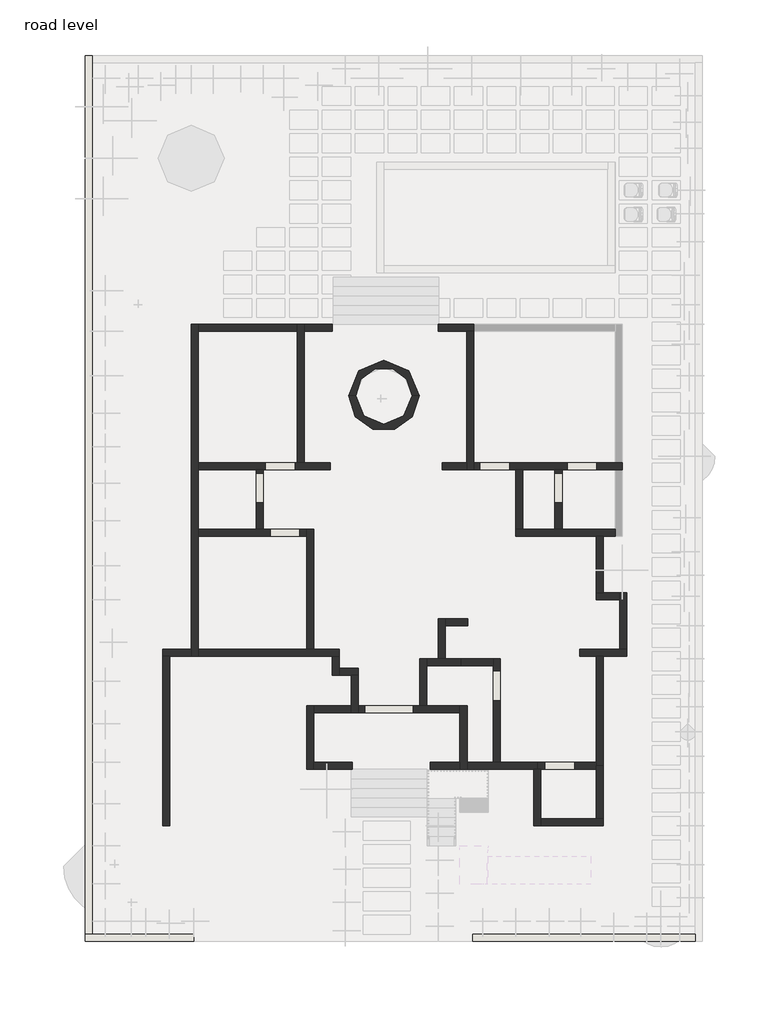
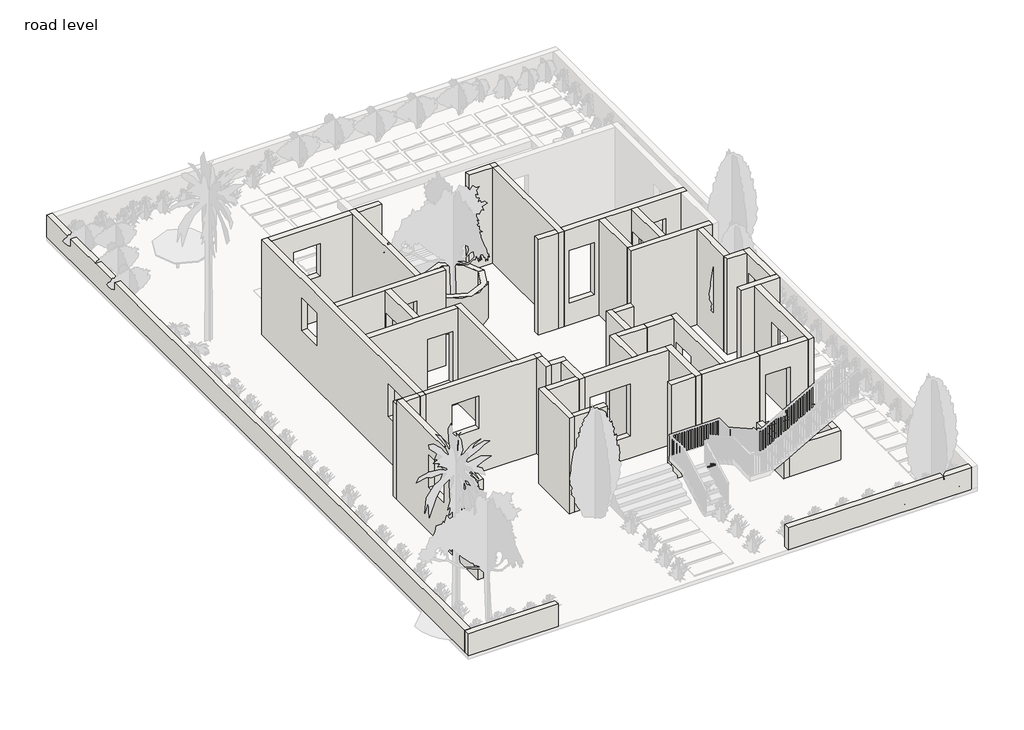
# One storey, part 1 of 5: 48 walls.
"""IFC4 building model written with IfcOpenShell, lengths in millimetres."""

from ifc_helpers import new_model, si_unit, point, frame, frame_2d, origin, origin_with_axes, place, context, project, spatial, polyline, circle_curve, trimmed, segment, composite_curve, outline, extrude, faceted_brep, element, save

model = new_model("IFC4")

# Units and contexts
model_context = context("Model", 3, world=origin())
ifc_project = project(units=[si_unit("LENGTHUNIT", "METRE", prefix="MILLI")], contexts=[model_context])

# Site, building, storey
site = spatial("IfcSite", under=ifc_project)
building = spatial("IfcBuilding", under=site)
storey = spatial("IfcBuildingStorey", under=building, Name="road level", Elevation=0.0)

# Walls
placement = place(None, origin())
element("IfcWall", 1, at=placement, inside=storey, context=model_context, shape_type="Brep", body=[
    faceted_brep([(-1469.5487175, 14534.2906886, 0.0), (-1469.5487175, 4018.6906886, 0.0), (-1469.5487175, 3790.0906886, 0.0), (-1469.5487175, 3790.0906886, 3962.4), (-1469.5487175, 4018.6906886, 3962.4), (-1469.5487175, 14534.2906886, 3962.4), (-1469.5487175, 5949.0906886, 3175.0), (-1469.5487175, 4907.6906886, 3175.0), (-1469.5487175, 4907.6906886, 1828.8), (-1469.5487175, 5949.0906886, 1828.8), (-1469.5487175, 11841.8906886, 3175.0), (-1469.5487175, 10800.4906886, 3175.0), (-1469.5487175, 10800.4906886, 1828.8), (-1469.5487175, 11841.8906886, 1828.8), (-1240.9487175, 14534.2906886, 0.0), (-1240.9487175, 14534.2906886, 3962.4), (-1240.9487175, 14305.6906886, 3962.4), (-1240.9487175, 10063.8906886, 3962.4), (-1240.9487175, 9835.2906886, 3962.4), (-1240.9487175, 7904.8906886, 3962.4), (-1240.9487175, 7676.2906886, 3962.4), (-1240.9487175, 4018.6906886, 3962.4), (-1240.9487175, 3790.0906886, 3962.4), (-1240.9487175, 3790.0906886, 0.0), (-1240.9487175, 4018.6906886, 0.0), (-1240.9487175, 7676.2906886, 0.0), (-1240.9487175, 7904.8906886, 0.0), (-1240.9487175, 9835.2906886, 0.0), (-1240.9487175, 10063.8906886, 0.0), (-1240.9487175, 14305.6906886, 0.0), (-1240.9487175, 5949.0906886, 3175.0), (-1240.9487175, 5949.0906886, 1828.8), (-1240.9487175, 4907.6906886, 1828.8), (-1240.9487175, 4907.6906886, 3175.0), (-1240.9487175, 11841.8906886, 3175.0), (-1240.9487175, 11841.8906886, 1828.8), (-1240.9487175, 10800.4906886, 1828.8), (-1240.9487175, 10800.4906886, 3175.0)], [[[0, 1, 2, 3, 4, 5], [6, 7, 8, 9], [10, 11, 12, 13]], [[14, 15, 16, 17, 18, 19, 20, 21, 22, 23, 24, 25, 26, 27, 28, 29], [30, 31, 32, 33], [34, 35, 36, 37]], [[2, 1, 0, 14, 29, 28, 27, 26, 25, 24, 23]], [[0, 5, 15, 14]], [[3, 2, 23, 22]], [[4, 3, 22, 21]], [[5, 4, 21, 20, 19, 18, 17, 16, 15]], [[31, 30, 6, 9]], [[32, 31, 9, 8]], [[33, 32, 8, 7]], [[30, 33, 7, 6]], [[35, 34, 10, 13]], [[36, 35, 13, 12]], [[37, 36, 12, 11]], [[34, 37, 11, 10]]]),
])
element("IfcWall", 2, at=placement, inside=storey, context=model_context, shape_type="Brep", body=[
    faceted_brep([(-1240.9487175, 9835.2906886, 0.0), (638.6512825, 9835.2906886, 0.0), (867.2512825, 9835.2906886, 0.0), (3034.6723193, 9835.2906886, 0.0), (3034.6723193, 9835.2906886, 3962.4), (867.2512825, 9835.2906886, 3962.4), (638.6512825, 9835.2906886, 3962.4), (-1240.9487175, 9835.2906886, 3962.4), (1895.9512825, 9835.2906886, 3073.4), (1895.9512825, 9835.2906886, 914.4), (930.7512825, 9835.2906886, 914.4), (930.7512825, 9835.2906886, 3073.4), (3034.6723193, 10063.8906886, 0.0), (2188.0512825, 10063.8906886, 0.0), (1959.4512825, 10063.8906886, 0.0), (-1240.9487175, 10063.8906886, 0.0), (-1240.9487175, 10063.8906886, 3962.4), (1959.4512825, 10063.8906886, 3962.4), (2188.0512825, 10063.8906886, 3962.4), (3034.6723193, 10063.8906886, 3962.4), (1895.9512825, 10063.8906886, 914.4), (1895.9512825, 10063.8906886, 3073.4), (930.7512825, 10063.8906886, 3073.4), (930.7512825, 10063.8906886, 914.4)], [[[0, 1, 2, 3, 4, 5, 6, 7], [8, 9, 10, 11]], [[12, 13, 14, 15, 16, 17, 18, 19], [20, 21, 22, 23]], [[3, 2, 1, 0, 15, 14, 13, 12]], [[4, 3, 12, 19]], [[0, 7, 16, 15]], [[20, 9, 8, 21]], [[21, 8, 11, 22]], [[22, 11, 10, 23]], [[9, 20, 23, 10]], [[16, 7, 6, 5, 4, 19, 18, 17]]]),
])
element("IfcWall", 3, at=placement, inside=storey, context=model_context, shape_type="Brep", body=[
    faceted_brep([(2188.0512825, 10063.8906886, 0.0), (2188.0512825, 14305.6906886, 0.0), (2188.0512825, 14534.2906886, 0.0), (2188.0512825, 14534.2906886, 3962.4), (2188.0512825, 14305.6906886, 3962.4), (2188.0512825, 10063.8906886, 3962.4), (1959.4512825, 10063.8906886, 0.0), (1959.4512825, 10063.8906886, 3962.4), (1959.4512825, 14305.6906886, 3962.4), (1959.4512825, 14534.2906886, 3962.4), (1959.4512825, 14534.2906886, 0.0), (1959.4512825, 14305.6906886, 0.0)], [[[0, 1, 2, 3, 4, 5]], [[6, 7, 8, 9, 10, 11]], [[2, 1, 0, 6, 11, 10]], [[0, 5, 7, 6]], [[3, 2, 10, 9]], [[5, 4, 3, 9, 8, 7]]]),
])
element("IfcWall", 4, at=placement, inside=storey, context=model_context, shape_type="SweptSolid", body=[
    extrude(outline(polyline([(0.0, 1959.4512825), (3962.4, 1959.4512825), (3962.4, -1240.9487175), (0.0, -1240.9487175), (0.0, 1959.4512825)]), holes=[polyline([(3175.0, 689.4512825), (1828.8, 689.4512825), (1828.8, -351.9487175), (3175.0, -351.9487175), (3175.0, 689.4512825)])]), frame((0.0, 14305.6906886, 0.0), z_axis=(0.0, 1.0, 0.0), x_axis=(0.0, 0.0, 1.0)), (0.0, 0.0, 1.0), 228.6),
])
element("IfcWall", 5, at=placement, inside=storey, context=model_context, shape_type="SweptSolid", body=[
    extrude(outline(polyline([(3102.4512825, 14305.6906886), (2188.0512825, 14305.6906886), (2188.0512825, 14534.2906886), (3102.4512825, 14534.2906886), (3102.4512825, 14305.6906886)])), origin_with_axes(), (0.0, 0.0, 1.0), 3962.4),
])
element("IfcWall", 6, at=placement, inside=storey, context=model_context, shape_type="Brep", body=[
    faceted_brep([(7445.8512825, 14305.6906886, 0.0), (7445.8512825, 10063.8906886, 0.0), (7445.8512825, 9835.2906886, 0.0), (7445.8512825, 9835.2906886, 3962.4), (7445.8512825, 10063.8906886, 3962.4), (7445.8512825, 14305.6906886, 3962.4), (7674.4512825, 14305.6906886, 0.0), (7674.4512825, 14305.6906886, 3962.4), (7674.4512825, 10063.8906886, 3962.4), (7674.4512825, 9835.2906886, 3962.4), (7674.4512825, 9835.2906886, 0.0), (7674.4512825, 10063.8906886, 0.0)], [[[0, 1, 2, 3, 4, 5]], [[6, 7, 8, 9, 10, 11]], [[2, 1, 0, 6, 11, 10]], [[0, 5, 7, 6]], [[3, 2, 10, 9]], [[5, 4, 3, 9, 8, 7]]]),
])
element("IfcWall", 7, at=placement, inside=storey, context=model_context, shape_type="Brep", body=[
    faceted_brep([(7674.4512825, 9835.2906886, 0.0), (9033.3512825, 9835.2906886, 0.0), (9261.9512825, 9835.2906886, 0.0), (10303.3512825, 9835.2906886, 0.0), (10531.9512825, 9835.2906886, 0.0), (12246.4512825, 9835.2906886, 0.0), (12475.0512825, 9835.2906886, 0.0), (12475.0512825, 9835.2906886, 3962.4), (12246.4512825, 9835.2906886, 3962.4), (10531.9512825, 9835.2906886, 3962.4), (10303.3512825, 9835.2906886, 3962.4), (9261.9512825, 9835.2906886, 3962.4), (9033.3512825, 9835.2906886, 3962.4), (7674.4512825, 9835.2906886, 3962.4), (10697.0512825, 9835.2906886, 914.4), (10697.0512825, 9835.2906886, 3073.4), (11662.2512825, 9835.2906886, 3073.4), (11662.2512825, 9835.2906886, 914.4), (7877.6512825, 9835.2906886, 914.4), (7877.6512825, 9835.2906886, 3073.4), (8842.8512825, 9835.2906886, 3073.4), (8842.8512825, 9835.2906886, 914.4), (12475.0512825, 10063.8906886, 0.0), (12246.4512825, 10063.8906886, 0.0), (7674.4512825, 10063.8906886, 0.0), (7674.4512825, 10063.8906886, 3962.4), (12246.4512825, 10063.8906886, 3962.4), (12475.0512825, 10063.8906886, 3962.4), (10697.0512825, 10063.8906886, 3073.4), (10697.0512825, 10063.8906886, 914.4), (11662.2512825, 10063.8906886, 914.4), (11662.2512825, 10063.8906886, 3073.4), (7877.6512825, 10063.8906886, 3073.4), (7877.6512825, 10063.8906886, 914.4), (8842.8512825, 10063.8906886, 914.4), (8842.8512825, 10063.8906886, 3073.4)], [[[0, 1, 2, 3, 4, 5, 6, 7, 8, 9, 10, 11, 12, 13], [14, 15, 16, 17], [18, 19, 20, 21]], [[22, 23, 24, 25, 26, 27], [28, 29, 30, 31], [32, 33, 34, 35]], [[6, 5, 4, 3, 2, 1, 0, 24, 23, 22]], [[0, 13, 25, 24]], [[7, 6, 22, 27]], [[14, 29, 28, 15]], [[15, 28, 31, 16]], [[30, 17, 16, 31]], [[29, 14, 17, 30]], [[18, 33, 32, 19]], [[19, 32, 35, 20]], [[20, 35, 34, 21]], [[33, 18, 21, 34]], [[13, 12, 11, 10, 9, 8, 7, 27, 26, 25]]]),
])
element("IfcWall", 8, at=placement, inside=storey, context=model_context, shape_type="Brep", body=[
    faceted_brep([(-1240.9487175, 7676.2906886, 0.0), (2264.2512825, 7676.2906886, 0.0), (2264.2512825, 7676.2906886, 3962.4), (-1240.9487175, 7676.2906886, 3962.4), (2048.3512825, 7676.2906886, 3073.4), (2048.3512825, 7676.2906886, 914.4), (1083.1512825, 7676.2906886, 914.4), (1083.1512825, 7676.2906886, 3073.4), (2264.2512825, 7904.8906886, 0.0), (867.2512825, 7904.8906886, 0.0), (638.6512825, 7904.8906886, 0.0), (-1240.9487175, 7904.8906886, 0.0), (-1240.9487175, 7904.8906886, 3962.4), (638.6512825, 7904.8906886, 3962.4), (867.2512825, 7904.8906886, 3962.4), (2264.2512825, 7904.8906886, 3962.4), (2048.3512825, 7904.8906886, 914.4), (2048.3512825, 7904.8906886, 3073.4), (1083.1512825, 7904.8906886, 3073.4), (1083.1512825, 7904.8906886, 914.4)], [[[0, 1, 2, 3], [4, 5, 6, 7]], [[8, 9, 10, 11, 12, 13, 14, 15], [16, 17, 18, 19]], [[1, 0, 11, 10, 9, 8]], [[0, 3, 12, 11]], [[2, 1, 8, 15]], [[16, 5, 4, 17]], [[17, 4, 7, 18]], [[18, 7, 6, 19]], [[5, 16, 19, 6]], [[3, 2, 15, 14, 13, 12]]]),
])
element("IfcWall", 9, at=placement, inside=storey, context=model_context, shape_type="SweptSolid", body=[
    extrude(outline(polyline([(9835.2906886, 0.0), (7904.8906886, 0.0), (7904.8906886, 3962.4), (9835.2906886, 3962.4), (9835.2906886, 0.0)]), holes=[polyline([(9720.9906886, 914.4), (9720.9906886, 3073.4), (8755.7906886, 3073.4), (8755.7906886, 914.4), (9720.9906886, 914.4)])]), frame((638.6512825, 0.0, 0.0), z_axis=(1.0, 0.0, 0.0), x_axis=(0.0, 1.0, 0.0)), (0.0, 0.0, 1.0), 228.6),
])
element("IfcWall", 10, at=placement, inside=storey, context=model_context, shape_type="Brep", body=[
    faceted_brep([(12246.4512825, 7904.8906886, 0.0), (10531.9512825, 7904.8906886, 0.0), (10303.3512825, 7904.8906886, 0.0), (9261.9512825, 7904.8906886, 0.0), (9033.3512825, 7904.8906886, 0.0), (9033.3512825, 7904.8906886, 3962.4), (9261.9512825, 7904.8906886, 3962.4), (10303.3512825, 7904.8906886, 3962.4), (10531.9512825, 7904.8906886, 3962.4), (12246.4512825, 7904.8906886, 3962.4), (12246.4512825, 7676.2906886, 0.0), (12246.4512825, 7676.2906886, 3962.4), (11865.4512825, 7676.2906886, 3962.4), (11636.8512825, 7676.2906886, 3962.4), (9033.3512825, 7676.2906886, 3962.4), (9033.3512825, 7676.2906886, 0.0), (11636.8512825, 7676.2906886, 0.0), (11865.4512825, 7676.2906886, 0.0)], [[[0, 1, 2, 3, 4, 5, 6, 7, 8, 9]], [[10, 11, 12, 13, 14, 15, 16, 17]], [[4, 3, 2, 1, 0, 10, 17, 16, 15]], [[0, 9, 11, 10]], [[5, 4, 15, 14]], [[9, 8, 7, 6, 5, 14, 13, 12, 11]]]),
])
element("IfcWall", 11, at=placement, inside=storey, context=model_context, shape_type="SweptSolid", body=[
    extrude(outline(polyline([(9835.2906886, 0.0), (7904.8906886, 0.0), (7904.8906886, 3962.4), (9835.2906886, 3962.4), (9835.2906886, 0.0)]), holes=[polyline([(9720.9906886, 914.4), (9720.9906886, 3073.4), (8755.7906886, 3073.4), (8755.7906886, 914.4), (9720.9906886, 914.4)])]), frame((10303.3512825, 0.0, 0.0), z_axis=(1.0, 0.0, 0.0), x_axis=(0.0, 1.0, 0.0)), (0.0, 0.0, 1.0), 228.6),
])
element("IfcWall", 12, at=placement, inside=storey, context=model_context, shape_type="SweptSolid", body=[
    extrude(outline(polyline([(9261.9512825, 9835.2906886), (9261.9512825, 7904.8906886), (9033.3512825, 7904.8906886), (9033.3512825, 9835.2906886), (9261.9512825, 9835.2906886)])), origin_with_axes(), (0.0, 0.0, 1.0), 3962.4),
])
element("IfcWall", 13, at=placement, inside=storey, context=model_context, shape_type="Brep", body=[
    faceted_brep([(-1240.9487175, 3790.0906886, 0.0), (3102.4512825, 3790.0906886, 0.0), (3331.0512825, 3790.0906886, 0.0), (3331.0512825, 3790.0906886, 3962.4), (3102.4512825, 3790.0906886, 3962.4), (-1240.9487175, 3790.0906886, 3962.4), (-199.5487175, 3790.0906886, 3175.0), (841.8512825, 3790.0906886, 3175.0), (841.8512825, 3790.0906886, 1828.8), (-199.5487175, 3790.0906886, 1828.8), (-1240.9487175, 4018.6906886, 0.0), (-1240.9487175, 4018.6906886, 3962.4), (2264.2512825, 4018.6906886, 3962.4), (2492.8512825, 4018.6906886, 3962.4), (3102.4512825, 4018.6906886, 3962.4), (3331.0512825, 4018.6906886, 3962.4), (3331.0512825, 4018.6906886, 0.0), (2492.8512825, 4018.6906886, 0.0), (2264.2512825, 4018.6906886, 0.0), (-199.5487175, 4018.6906886, 3175.0), (-199.5487175, 4018.6906886, 1828.8), (841.8512825, 4018.6906886, 1828.8), (841.8512825, 4018.6906886, 3175.0)], [[[0, 1, 2, 3, 4, 5], [6, 7, 8, 9]], [[10, 11, 12, 13, 14, 15, 16, 17, 18], [19, 20, 21, 22]], [[2, 1, 0, 10, 18, 17, 16]], [[0, 5, 11, 10]], [[3, 2, 16, 15]], [[5, 4, 14, 13, 12, 11]], [[4, 3, 15, 14]], [[20, 19, 6, 9]], [[21, 20, 9, 8]], [[22, 21, 8, 7]], [[19, 22, 7, 6]]]),
])
element("IfcWall", 14, at=placement, inside=storey, context=model_context, shape_type="Brep", body=[
    faceted_brep([(2492.8512825, 4018.6906886, 0.0), (2492.8512825, 7904.8906886, 0.0), (2492.8512825, 7904.8906886, 3962.4), (2492.8512825, 4018.6906886, 3962.4), (2264.2512825, 4018.6906886, 0.0), (2264.2512825, 4018.6906886, 3962.4), (2264.2512825, 7676.2906886, 3962.4), (2264.2512825, 7904.8906886, 3962.4), (2264.2512825, 7904.8906886, 0.0), (2264.2512825, 7676.2906886, 0.0)], [[[0, 1, 2, 3]], [[4, 5, 6, 7, 8, 9]], [[1, 0, 4, 9, 8]], [[0, 3, 5, 4]], [[2, 1, 8, 7]], [[3, 2, 7, 6, 5]]]),
])
element("IfcWall", 15, at=placement, inside=storey, context=model_context, shape_type="Brep", body=[
    faceted_brep([(3102.4512825, 3790.0906886, 0.0), (3102.4512825, 3180.4906886, 0.0), (3102.4512825, 3180.4906886, 3962.4), (3102.4512825, 3790.0906886, 3962.4), (3331.0512825, 3790.0906886, 0.0), (3331.0512825, 3790.0906886, 3962.4), (3331.0512825, 3409.0906886, 3962.4), (3331.0512825, 3180.4906886, 3962.4), (3331.0512825, 3180.4906886, 0.0), (3331.0512825, 3409.0906886, 0.0)], [[[0, 1, 2, 3]], [[4, 5, 6, 7, 8, 9]], [[1, 0, 4, 9, 8]], [[0, 3, 5, 4]], [[2, 1, 8, 7]], [[3, 2, 7, 6, 5]]]),
])
element("IfcWall", 16, at=placement, inside=storey, context=model_context, shape_type="Brep", body=[
    faceted_brep([(3331.0512825, 3180.4906886, 0.0), (3712.0512825, 3180.4906886, 0.0), (3940.6512825, 3180.4906886, 0.0), (3940.6512825, 3180.4906886, 3962.4), (3712.0512825, 3180.4906886, 3962.4), (3331.0512825, 3180.4906886, 3962.4), (3331.0512825, 3409.0906886, 0.0), (3331.0512825, 3409.0906886, 3962.4), (3940.6512825, 3409.0906886, 3962.4), (3940.6512825, 3409.0906886, 0.0)], [[[0, 1, 2, 3, 4, 5]], [[6, 7, 8, 9]], [[2, 1, 0, 6, 9]], [[0, 5, 7, 6]], [[3, 2, 9, 8]], [[5, 4, 3, 8, 7]]]),
])
element("IfcWall", 17, at=placement, inside=storey, context=model_context, shape_type="Brep", body=[
    faceted_brep([(3712.0512825, 3180.4906886, 0.0), (3712.0512825, 2189.8906886, 0.0), (3712.0512825, 1961.2906886, 0.0), (3712.0512825, 1961.2906886, 3962.4), (3712.0512825, 2189.8906886, 3962.4), (3712.0512825, 3180.4906886, 3962.4), (3940.6512825, 3180.4906886, 0.0), (3940.6512825, 3180.4906886, 3962.4), (3940.6512825, 2189.8906886, 3962.4), (3940.6512825, 1961.2906886, 3962.4), (3940.6512825, 1961.2906886, 0.0), (3940.6512825, 2189.8906886, 0.0)], [[[0, 1, 2, 3, 4, 5]], [[6, 7, 8, 9, 10, 11]], [[2, 1, 0, 6, 11, 10]], [[0, 5, 7, 6]], [[3, 2, 10, 9]], [[5, 4, 3, 9, 8, 7]]]),
])
element("IfcWall", 18, at=placement, inside=storey, context=model_context, shape_type="Brep", body=[
    faceted_brep([(3940.6512825, 1961.2906886, 0.0), (7229.9512825, 1961.2906886, 0.0), (7229.9512825, 1961.2906886, 3962.4), (3940.6512825, 1961.2906886, 3962.4), (5718.6512825, 1961.2906886, 3073.4), (5718.6512825, 1961.2906886, 914.4), (4143.8512825, 1961.2906886, 914.4), (4143.8512825, 1961.2906886, 3073.4), (7229.9512825, 2189.8906886, 0.0), (6150.4512825, 2189.8906886, 0.0), (5921.8512825, 2189.8906886, 0.0), (3940.6512825, 2189.8906886, 0.0), (3940.6512825, 2189.8906886, 3962.4), (5921.8512825, 2189.8906886, 3962.4), (6150.4512825, 2189.8906886, 3962.4), (7229.9512825, 2189.8906886, 3962.4), (5718.6512825, 2189.8906886, 914.4), (5718.6512825, 2189.8906886, 3073.4), (4143.8512825, 2189.8906886, 3073.4), (4143.8512825, 2189.8906886, 914.4)], [[[0, 1, 2, 3], [4, 5, 6, 7]], [[8, 9, 10, 11, 12, 13, 14, 15], [16, 17, 18, 19]], [[1, 0, 11, 10, 9, 8]], [[0, 3, 12, 11]], [[2, 1, 8, 15]], [[16, 5, 4, 17]], [[17, 4, 7, 18]], [[18, 7, 6, 19]], [[5, 16, 19, 6]], [[3, 2, 15, 14, 13, 12]]]),
])
element("IfcWall", 19, at=placement, inside=storey, context=model_context, shape_type="Brep", body=[
    faceted_brep([(6150.4512825, 2189.8906886, 0.0), (6150.4512825, 3485.2906886, 0.0), (6150.4512825, 3713.8906886, 0.0), (6150.4512825, 3713.8906886, 3962.4), (6150.4512825, 3485.2906886, 3962.4), (6150.4512825, 2189.8906886, 3962.4), (5921.8512825, 2189.8906886, 0.0), (5921.8512825, 2189.8906886, 3962.4), (5921.8512825, 3713.8906886, 3962.4), (5921.8512825, 3713.8906886, 0.0)], [[[0, 1, 2, 3, 4, 5]], [[6, 7, 8, 9]], [[2, 1, 0, 6, 9]], [[0, 5, 7, 6]], [[3, 2, 9, 8]], [[5, 4, 3, 8, 7]]]),
])
element("IfcWall", 20, at=placement, inside=storey, context=model_context, shape_type="Brep", body=[
    faceted_brep([(6150.4512825, 3485.2906886, 0.0), (7255.3512825, 3485.2906886, 0.0), (7255.3512825, 3485.2906886, 3962.4), (6150.4512825, 3485.2906886, 3962.4), (6150.4512825, 3713.8906886, 0.0), (6150.4512825, 3713.8906886, 3962.4), (6531.4512825, 3713.8906886, 3962.4), (6760.0512825, 3713.8906886, 3962.4), (7255.3512825, 3713.8906886, 3962.4), (7255.3512825, 3713.8906886, 0.0), (6760.0512825, 3713.8906886, 0.0), (6531.4512825, 3713.8906886, 0.0)], [[[0, 1, 2, 3]], [[4, 5, 6, 7, 8, 9, 10, 11]], [[1, 0, 4, 11, 10, 9]], [[2, 1, 9, 8]], [[0, 3, 5, 4]], [[3, 2, 8, 7, 6, 5]]]),
])
element("IfcWall", 21, at=placement, inside=storey, context=model_context, shape_type="Brep", body=[
    faceted_brep([(6760.0512825, 3713.8906886, 0.0), (6760.0512825, 4780.6906886, 0.0), (6760.0512825, 5009.2906886, 0.0), (6760.0512825, 5009.2906886, 3962.4), (6760.0512825, 4780.6906886, 3962.4), (6760.0512825, 3713.8906886, 3962.4), (6531.4512825, 3713.8906886, 0.0), (6531.4512825, 3713.8906886, 3962.4), (6531.4512825, 5009.2906886, 3962.4), (6531.4512825, 5009.2906886, 0.0)], [[[0, 1, 2, 3, 4, 5]], [[6, 7, 8, 9]], [[2, 1, 0, 6, 9]], [[3, 2, 9, 8]], [[0, 5, 7, 6]], [[5, 4, 3, 8, 7]]]),
])
element("IfcWall", 22, at=placement, inside=storey, context=model_context, shape_type="SweptSolid", body=[
    extrude(outline(polyline([(7483.9512825, 4780.6906886), (6760.0512825, 4780.6906886), (6760.0512825, 5009.2906886), (7483.9512825, 5009.2906886), (7483.9512825, 4780.6906886)])), origin_with_axes(), (0.0, 0.0, 1.0), 3962.4),
])
element("IfcWall", 23, at=placement, inside=storey, context=model_context, shape_type="Brep", body=[
    faceted_brep([(7229.9512825, 2189.8906886, 0.0), (7229.9512825, 1961.2906886, 0.0), (7229.9512825, 361.0906886, 0.0), (7229.9512825, 132.4906886, 0.0), (7229.9512825, 132.4906886, 3962.4), (7229.9512825, 361.0906886, 3962.4), (7229.9512825, 1961.2906886, 3962.4), (7229.9512825, 2189.8906886, 3962.4), (7458.5512825, 2189.8906886, 0.0), (7458.5512825, 2189.8906886, 3962.4), (7458.5512825, 361.0906886, 3962.4), (7458.5512825, 132.4906886, 3962.4), (7458.5512825, 132.4906886, 0.0), (7458.5512825, 361.0906886, 0.0)], [[[0, 1, 2, 3, 4, 5, 6, 7]], [[8, 9, 10, 11, 12, 13]], [[3, 2, 1, 0, 8, 13, 12]], [[4, 3, 12, 11]], [[0, 7, 9, 8]], [[7, 6, 5, 4, 11, 10, 9]]]),
])
element("IfcWall", 24, at=placement, inside=storey, context=model_context, shape_type="SweptSolid", body=[
    extrude(outline(polyline([(6264.7512825, 361.0906886), (7229.9512825, 361.0906886), (7229.9512825, 132.4906886), (6264.7512825, 132.4906886), (6264.7512825, 361.0906886)])), origin_with_axes(), (0.0, 0.0, 1.0), 3962.4),
])
element("IfcWall", 25, at=placement, inside=storey, context=model_context, shape_type="Brep", body=[
    faceted_brep([(2264.2512825, 2189.8906886, 0.0), (2264.2512825, 132.4906886, 0.0), (2264.2512825, 132.4906886, 3962.4), (2264.2512825, 2189.8906886, 3962.4), (2492.8512825, 2189.8906886, 0.0), (2492.8512825, 2189.8906886, 3962.4), (2492.8512825, 1961.2906886, 3962.4), (2492.8512825, 361.0906886, 3962.4), (2492.8512825, 132.4906886, 3962.4), (2492.8512825, 132.4906886, 0.0), (2492.8512825, 361.0906886, 0.0), (2492.8512825, 1961.2906886, 0.0)], [[[0, 1, 2, 3]], [[4, 5, 6, 7, 8, 9, 10, 11]], [[1, 0, 4, 11, 10, 9]], [[2, 1, 9, 8]], [[0, 3, 5, 4]], [[3, 2, 8, 7, 6, 5]]]),
])
element("IfcWall", 26, at=placement, inside=storey, context=model_context, shape_type="SweptSolid", body=[
    extrude(outline(polyline([(3750.1512825, 132.4906886), (2492.8512825, 132.4906886), (2492.8512825, 361.0906886), (3750.1512825, 361.0906886), (3750.1512825, 132.4906886)])), origin_with_axes(), (0.0, 0.0, 1.0), 3962.4),
])
element("IfcWall", 27, at=placement, inside=storey, context=model_context, shape_type="SweptSolid", body=[
    extrude(outline(polyline([(2492.8512825, 2189.8906886), (3712.0512825, 2189.8906886), (3712.0512825, 1961.2906886), (2492.8512825, 1961.2906886), (2492.8512825, 2189.8906886)])), origin_with_axes(), (0.0, 0.0, 1.0), 3962.4),
])
element("IfcWall", 28, at=placement, inside=storey, context=model_context, shape_type="Brep", body=[
    faceted_brep([(7458.5512825, 132.4906886, 0.0), (9617.5512825, 132.4906886, 0.0), (9731.8512825, 132.4906886, 0.0), (9731.8512825, 132.4906886, 3962.4), (9617.5512825, 132.4906886, 3962.4), (7458.5512825, 132.4906886, 3962.4), (7458.5512825, 361.0906886, 0.0), (7458.5512825, 361.0906886, 3962.4), (8309.4512825, 361.0906886, 3962.4), (8538.0512825, 361.0906886, 3962.4), (9731.8512825, 361.0906886, 3962.4), (9731.8512825, 361.0906886, 0.0), (8538.0512825, 361.0906886, 0.0), (8309.4512825, 361.0906886, 0.0)], [[[0, 1, 2, 3, 4, 5]], [[6, 7, 8, 9, 10, 11, 12, 13]], [[2, 1, 0, 6, 13, 12, 11]], [[0, 5, 7, 6]], [[5, 4, 3, 10, 9, 8, 7]], [[2, 11, 10, 3]]]),
])
element("IfcWall", 29, at=placement, inside=storey, context=model_context, shape_type="Brep", body=[
    faceted_brep([(11636.8512825, 361.0906886, 0.0), (9731.8512825, 361.0906886, 0.0), (9731.8512825, 361.0906886, 3962.4), (11636.8512825, 361.0906886, 3962.4), (9973.1512825, 361.0906886, 3073.4), (9973.1512825, 361.0906886, 914.4), (10938.3512825, 361.0906886, 914.4), (10938.3512825, 361.0906886, 3073.4), (9731.8512825, 132.4906886, 0.0), (9846.1512825, 132.4906886, 0.0), (11636.8512825, 132.4906886, 0.0), (11636.8512825, 132.4906886, 1219.2), (11636.8512825, 132.4906886, 3962.4), (9731.8512825, 132.4906886, 3962.4), (9973.1512825, 132.4906886, 914.4), (9973.1512825, 132.4906886, 3073.4), (10938.3512825, 132.4906886, 3073.4), (10938.3512825, 132.4906886, 914.4), (11636.8512825, 246.7906886, 0.0)], [[[0, 1, 2, 3], [4, 5, 6, 7]], [[8, 9, 10, 11, 12, 13], [14, 15, 16, 17]], [[1, 0, 18, 10, 9, 8]], [[14, 5, 4, 15]], [[15, 4, 7, 16]], [[16, 7, 6, 17]], [[5, 14, 17, 6]], [[3, 2, 13, 12]], [[1, 8, 13, 2]], [[10, 18, 0, 3, 12, 11]]]),
])
element("IfcWall", 30, at=placement, inside=storey, context=model_context, shape_type="Brep", body=[
    faceted_brep([(12627.4512825, 4018.6906886, 0.0), (12398.8512825, 4018.6906886, 0.0), (11103.4512825, 4018.6906886, 0.0), (11103.4512825, 4018.6906886, 3962.4), (12398.8512825, 4018.6906886, 3962.4), (12627.4512825, 4018.6906886, 3962.4), (12627.4512825, 3790.0906886, 0.0), (12627.4512825, 3790.0906886, 3962.4), (11865.4512825, 3790.0906886, 3962.4), (11636.8512825, 3790.0906886, 3962.4), (11103.4512825, 3790.0906886, 3962.4), (11103.4512825, 3790.0906886, 0.0), (11636.8512825, 3790.0906886, 0.0), (11865.4512825, 3790.0906886, 0.0)], [[[0, 1, 2, 3, 4, 5]], [[6, 7, 8, 9, 10, 11, 12, 13]], [[2, 1, 0, 6, 13, 12, 11]], [[3, 2, 11, 10]], [[0, 5, 7, 6]], [[5, 4, 3, 10, 9, 8, 7]]]),
])
element("IfcWall", 31, at=placement, inside=storey, context=model_context, shape_type="Brep", body=[
    faceted_brep([(12627.4512825, 4018.6906886, 0.0), (12627.4512825, 5847.4906886, 0.0), (12627.4512825, 5847.4906886, 3962.4), (12627.4512825, 4018.6906886, 3962.4), (12627.4512825, 4450.4906886, 3175.0), (12627.4512825, 5491.8906886, 3175.0), (12627.4512825, 5491.8906886, 1828.8), (12627.4512825, 4450.4906886, 1828.8), (12398.8512825, 4018.6906886, 0.0), (12398.8512825, 4018.6906886, 3962.4), (12398.8512825, 5618.8906886, 3962.4), (12398.8512825, 5847.4906886, 3962.4), (12398.8512825, 5847.4906886, 0.0), (12398.8512825, 5618.8906886, 0.0), (12398.8512825, 4450.4906886, 3175.0), (12398.8512825, 4450.4906886, 1828.8), (12398.8512825, 5491.8906886, 1828.8), (12398.8512825, 5491.8906886, 3175.0), (12475.0512825, 4018.6906886, 3962.4), (12475.0512825, 5847.4906886, 3962.4)], [[[0, 1, 2, 3], [4, 5, 6, 7]], [[8, 9, 10, 11, 12, 13], [14, 15, 16, 17]], [[1, 0, 8, 13, 12]], [[0, 3, 18, 9, 8]], [[2, 1, 12, 11, 19]], [[19, 11, 10, 9, 18, 3, 2]], [[15, 14, 4, 7]], [[16, 15, 7, 6]], [[17, 16, 6, 5]], [[14, 17, 5, 4]]]),
])
element("IfcWall", 32, at=placement, inside=storey, context=model_context, shape_type="Brep", body=[
    faceted_brep([(12398.8512825, 5847.4906886, 0.0), (11865.4512825, 5847.4906886, 0.0), (11636.8512825, 5847.4906886, 0.0), (11636.8512825, 5847.4906886, 3962.4), (11865.4512825, 5847.4906886, 3962.4), (12398.8512825, 5847.4906886, 3962.4), (12398.8512825, 5618.8906886, 0.0), (12398.8512825, 5618.8906886, 3962.4), (11636.8512825, 5618.8906886, 3962.4), (11636.8512825, 5618.8906886, 0.0)], [[[0, 1, 2, 3, 4, 5]], [[6, 7, 8, 9]], [[2, 1, 0, 6, 9]], [[0, 5, 7, 6]], [[3, 2, 9, 8]], [[5, 4, 3, 8, 7]]]),
])
element("IfcWall", 33, at=placement, inside=storey, context=model_context, shape_type="SweptSolid", body=[
    extrude(outline(polyline([(11865.4512825, 7676.2906886), (11865.4512825, 5847.4906886), (11636.8512825, 5847.4906886), (11636.8512825, 7676.2906886), (11865.4512825, 7676.2906886)])), origin_with_axes(), (0.0, 0.0, 1.0), 3962.4),
])
element("IfcWall", 34, at=placement, inside=storey, context=model_context, shape_type="Brep", body=[
    faceted_brep([(-1469.5487175, 4018.6906886, 0.0), (-2383.9487175, 4018.6906886, 0.0), (-2383.9487175, 4018.6906886, 3962.4), (-1469.5487175, 4018.6906886, 3962.4), (-1469.5487175, 3790.0906886, 0.0), (-1469.5487175, 3790.0906886, 3962.4), (-2383.9487175, 3790.0906886, 3962.4), (-2383.9487175, 3790.0906886, 0.0), (-2155.3487175, 3790.0906886, 0.0)], [[[0, 1, 2, 3]], [[4, 5, 6, 7, 8]], [[1, 0, 4, 8, 7]], [[3, 2, 6, 5]], [[0, 3, 5, 4]], [[2, 1, 7, 6]]]),
])
element("IfcWall", 35, at=placement, inside=storey, context=model_context, shape_type="Brep", body=[
    faceted_brep([(-2383.9487175, 3790.0906886, 0.0), (-2383.9487175, -1696.3093114, 0.0), (-2383.9487175, -1696.3093114, 4114.8), (-2383.9487175, 3790.0906886, 4114.8), (-2383.9487175, 3790.0906886, 3962.4), (-2383.9487175, 1624.7406886, 3175.0), (-2383.9487175, 583.3406886, 3175.0), (-2383.9487175, 583.3406886, 1828.8), (-2383.9487175, 1624.7406886, 1828.8), (-2155.3487175, 3790.0906886, 0.0), (-2155.3487175, 3790.0906886, 4114.8), (-2155.3487175, -1696.3093114, 4114.8), (-2155.3487175, -1696.3093114, 0.0), (-2155.3487175, 1624.7406886, 3175.0), (-2155.3487175, 1624.7406886, 1828.8), (-2155.3487175, 583.3406886, 1828.8), (-2155.3487175, 583.3406886, 3175.0)], [[[0, 1, 2, 3, 4], [5, 6, 7, 8]], [[9, 10, 11, 12], [13, 14, 15, 16]], [[1, 0, 9, 12]], [[2, 1, 12, 11]], [[3, 2, 11, 10]], [[0, 4, 3, 10, 9]], [[14, 13, 5, 8]], [[15, 14, 8, 7]], [[16, 15, 7, 6]], [[13, 16, 6, 5]]]),
])
element("IfcWall", 36, at=placement, inside=storey, context=model_context, shape_type="SweptSolid", body=[
    extrude(outline(polyline([(6658.4512825, 10063.8906886), (7445.8512825, 10063.8906886), (7445.8512825, 9835.2906886), (6658.4512825, 9835.2906886), (6658.4512825, 10063.8906886)])), origin_with_axes(), (0.0, 0.0, 1.0), 3962.4),
])
element("IfcWall", 37, at=placement, inside=storey, context=model_context, shape_type="Brep", body=[
    faceted_brep([(6531.4512825, 14305.6906886, 0.0), (7445.8512825, 14305.6906886, 0.0), (7674.4512825, 14305.6906886, 0.0), (7674.4512825, 14305.6906886, 3962.4), (7445.8512825, 14305.6906886, 3962.4), (6531.4512825, 14305.6906886, 3962.4), (6531.4512825, 14534.2906886, 0.0), (6531.4512825, 14534.2906886, 3962.4), (7445.8512825, 14534.2906886, 3962.4), (7674.4512825, 14534.2906886, 3962.4), (7674.4512825, 14534.2906886, 0.0), (7445.8512825, 14331.0906886, 3962.4)], [[[0, 1, 2, 3, 4, 5]], [[6, 7, 8, 9, 10]], [[2, 1, 0, 6, 10]], [[0, 5, 7, 6]], [[3, 2, 10, 9]], [[5, 4, 11, 8, 7]], [[4, 3, 9, 8, 11]]]),
])
element("IfcWall", 38, at=placement, inside=storey, context=model_context, shape_type="Brep", body=[
    faceted_brep([(8538.0512825, 361.0906886, 0.0), (8538.0512825, 3713.8906886, 0.0), (8538.0512825, 3713.8906886, 3962.4), (8538.0512825, 361.0906886, 3962.4), (8538.0512825, 3320.1906886, 3073.4), (8538.0512825, 3320.1906886, 914.4), (8538.0512825, 2354.9906886, 914.4), (8538.0512825, 2354.9906886, 3073.4), (8309.4512825, 3713.8906886, 0.0), (8309.4512825, 3485.2906886, 0.0), (8309.4512825, 361.0906886, 0.0), (8309.4512825, 361.0906886, 3962.4), (8309.4512825, 3485.2906886, 3962.4), (8309.4512825, 3713.8906886, 3962.4), (8309.4512825, 3320.1906886, 914.4), (8309.4512825, 3320.1906886, 3073.4), (8309.4512825, 2354.9906886, 3073.4), (8309.4512825, 2354.9906886, 914.4)], [[[0, 1, 2, 3], [4, 5, 6, 7]], [[8, 9, 10, 11, 12, 13], [14, 15, 16, 17]], [[1, 0, 10, 9, 8]], [[0, 3, 11, 10]], [[2, 1, 8, 13]], [[14, 5, 4, 15]], [[15, 4, 7, 16]], [[16, 7, 6, 17]], [[5, 14, 17, 6]], [[3, 2, 13, 12, 11]]]),
])
element("IfcWall", 39, at=placement, inside=storey, context=model_context, shape_type="SweptSolid", body=[
    extrude(outline(polyline([(7255.3512825, 3713.8906886), (8309.4512825, 3713.8906886), (8309.4512825, 3485.2906886), (7255.3512825, 3485.2906886), (7255.3512825, 3713.8906886)])), origin_with_axes(), (0.0, 0.0, 1.0), 3962.4),
])
element("IfcWall", 40, at=placement, inside=storey, context=model_context, shape_type="SweptSolid", body=[
    extrude(outline(polyline([(7636.3512825, -5201.5093114), (14837.2512825, -5201.5093114), (14837.2512825, -5430.1093114), (7636.3512825, -5430.1093114), (7636.3512825, -5201.5093114)])), origin_with_axes(), (0.0, 0.0, 1.0), 914.4),
])
element("IfcWall", 41, at=placement, inside=storey, context=model_context, shape_type="Brep", body=[
    faceted_brep([(-4669.9487175, -5201.5093114, 0.0), (-4669.9487175, 22992.4906886, 0.0), (-4669.9487175, 23221.0906886, 0.0), (-4669.9487175, 23221.0906886, 914.4), (-4669.9487175, 22992.4906886, 914.4), (-4669.9487175, -5201.5093114, 914.4), (-4898.5487175, -5201.5093114, 0.0), (-4898.5487175, -5201.5093114, 914.4), (-4898.5487175, 23221.0906886, 914.4), (-4898.5487175, 23221.0906886, 0.0)], [[[0, 1, 2, 3, 4, 5]], [[6, 7, 8, 9]], [[2, 1, 0, 6, 9]], [[5, 4, 3, 8, 7]], [[0, 5, 7, 6]], [[3, 2, 9, 8]]]),
])
element("IfcWall", 42, at=placement, inside=storey, context=model_context, shape_type="Brep", body=[
    faceted_brep([(-1380.6487175, -5201.5093114, 0.0), (-4669.9487175, -5201.5093114, 0.0), (-4898.5487175, -5201.5093114, 0.0), (-4898.5487175, -5201.5093114, 914.4), (-4669.9487175, -5201.5093114, 914.4), (-1380.6487175, -5201.5093114, 914.4), (-1380.6487175, -5430.1093114, 0.0), (-1380.6487175, -5430.1093114, 914.4), (-4898.5487175, -5430.1093114, 914.4), (-4898.5487175, -5430.1093114, 0.0)], [[[0, 1, 2, 3, 4, 5]], [[6, 7, 8, 9]], [[2, 1, 0, 6, 9]], [[5, 4, 3, 8, 7]], [[0, 5, 7, 6]], [[3, 2, 9, 8]]]),
])
element("IfcWall", 43, at=placement, inside=storey, context=model_context, shape_type="SweptSolid", body=[
    extrude(outline(composite_curve([segment(polyline([(3851.3160064, 12224.5614263), (3622.7160064, 12224.5614263)]), True, "CONTINUOUS"), segment(trimmed(circle_curve(frame_2d((4765.7160064, 12224.5614263)), 1143.0), [point((3622.7160064, 12224.5614263))], [point((5908.7160064, 12224.5614263))], False, "CARTESIAN"), True, "CONTINUOUS"), segment(polyline([(5908.7160064, 12224.5614263), (5680.1160064, 12224.5614263)]), True, "CONTINUOUS"), segment(trimmed(circle_curve(frame_2d((4765.7160064, 12224.5614263)), 914.4), [point((5680.1160064, 12224.5614263))], [point((3851.3160064, 12224.5614263))], True, "CARTESIAN"), True, "CONTINUOUS")], self_intersect=False)), origin_with_axes(), (0.0, 0.0, 1.0), 1524.0),
])
element("IfcWall", 44, at=placement, inside=storey, context=model_context, shape_type="SweptSolid", body=[
    extrude(outline(composite_curve([segment(polyline([(5680.1160064, 12224.5614263), (5908.7160064, 12224.5614263)]), True, "CONTINUOUS"), segment(trimmed(circle_curve(frame_2d((4765.7160064, 12224.5614263)), 1143.0), [point((5908.7160064, 12224.5614263))], [point((3622.7160064, 12224.5614263))], False, "CARTESIAN"), True, "CONTINUOUS"), segment(polyline([(3622.7160064, 12224.5614263), (3851.3160064, 12224.5614263)]), True, "CONTINUOUS"), segment(trimmed(circle_curve(frame_2d((4765.7160064, 12224.5614263)), 914.4), [point((3851.3160064, 12224.5614263))], [point((5680.1160064, 12224.5614263))], True, "CARTESIAN"), True, "CONTINUOUS")], self_intersect=False)), origin_with_axes(), (0.0, 0.0, 1.0), 1524.0),
])
element("IfcWall", 45, at=placement, inside=storey, context=model_context, shape_type="Brep", body=[
    faceted_brep([(9617.5512825, 132.4906886, 0.0), (9617.5512825, -1696.3093114, 0.0), (9617.5512825, -1696.3093114, 1219.2), (9617.5512825, 132.4906886, 1219.2), (9846.1512825, 132.4906886, 0.0), (9846.1512825, 132.4906886, 1219.2), (9846.1512825, -1467.7093114, 1219.2), (9846.1512825, -1696.3093114, 1219.2), (9846.1512825, -1696.3093114, 0.0), (9846.1512825, -1467.7093114, 0.0), (9731.8512825, 132.4906886, 0.0)], [[[0, 1, 2, 3]], [[4, 5, 6, 7, 8, 9]], [[1, 0, 10, 4, 9, 8]], [[3, 2, 7, 6, 5]], [[0, 3, 5, 4, 10]], [[2, 1, 8, 7]]]),
])
element("IfcWall", 46, at=placement, inside=storey, context=model_context, shape_type="Brep", body=[
    faceted_brep([(9846.1512825, -1696.3093114, 0.0), (11865.4512825, -1696.3093114, 0.0), (11865.4512825, -1696.3093114, 1219.2), (9846.1512825, -1696.3093114, 1219.2), (9846.1512825, -1467.7093114, 0.0), (9846.1512825, -1467.7093114, 1219.2), (11636.8512825, -1467.7093114, 1219.2), (11865.4512825, -1467.7093114, 1219.2), (11865.4512825, -1467.7093114, 0.0), (11636.8512825, -1467.7093114, 0.0)], [[[0, 1, 2, 3]], [[4, 5, 6, 7, 8, 9]], [[1, 0, 4, 9, 8]], [[3, 2, 7, 6, 5]], [[0, 3, 5, 4]], [[2, 1, 8, 7]]]),
])
element("IfcWall", 47, at=placement, inside=storey, context=model_context, shape_type="Brep", body=[
    faceted_brep([(11865.4512825, -1467.7093114, 0.0), (11865.4512825, 246.7906886, 0.0), (11865.4512825, 246.7906886, 1219.2), (11865.4512825, 132.4906886, 1219.2), (11865.4512825, -1467.7093114, 1219.2), (11636.8512825, -1467.7093114, 0.0), (11636.8512825, -1467.7093114, 1219.2), (11636.8512825, 132.4906886, 1219.2), (11636.8512825, 246.7906886, 1219.2), (11636.8512825, 246.7906886, 0.0), (11636.8512825, 132.4906886, 0.0)], [[[0, 1, 2, 3, 4]], [[5, 6, 7, 8, 9, 10]], [[1, 0, 5, 10, 9]], [[2, 1, 9, 8]], [[4, 3, 2, 8, 7, 6]], [[0, 4, 6, 5]]]),
])
element("IfcWall", 48, at=placement, inside=storey, context=model_context, shape_type="Brep", body=[
    faceted_brep([(11865.4512825, 246.7906886, 0.0), (11865.4512825, 3790.0906886, 0.0), (11865.4512825, 3790.0906886, 3962.4), (11865.4512825, 132.4906886, 3962.4), (11865.4512825, 132.4906886, 1219.2), (11865.4512825, 246.7906886, 1219.2), (11865.4512825, 1554.8906886, 3175.0), (11865.4512825, 2596.2906886, 3175.0), (11865.4512825, 2596.2906886, 1828.8), (11865.4512825, 1554.8906886, 1828.8), (11636.8512825, 246.7906886, 0.0), (11636.8512825, 246.7906886, 1219.2), (11636.8512825, 132.4906886, 1219.2), (11636.8512825, 132.4906886, 3962.4), (11636.8512825, 361.0906886, 3962.4), (11636.8512825, 3790.0906886, 3962.4), (11636.8512825, 3790.0906886, 0.0), (11636.8512825, 361.0906886, 0.0), (11636.8512825, 1554.8906886, 3175.0), (11636.8512825, 1554.8906886, 1828.8), (11636.8512825, 2596.2906886, 1828.8), (11636.8512825, 2596.2906886, 3175.0)], [[[0, 1, 2, 3, 4, 5], [6, 7, 8, 9]], [[10, 11, 12, 13, 14, 15, 16, 17], [18, 19, 20, 21]], [[1, 0, 10, 17, 16]], [[2, 1, 16, 15]], [[0, 5, 11, 10]], [[4, 12, 11, 5]], [[4, 3, 13, 12]], [[3, 2, 15, 14, 13]], [[19, 18, 6, 9]], [[20, 19, 9, 8]], [[21, 20, 8, 7]], [[18, 21, 7, 6]]]),
])

save(model, "model.ifc")

# Revit data of these elements
# Type
#   Assembly Code = "B2010"
#   Layers, outside or top first: 0' - 9" no material (function 1)
# Elements 1, 2, 3, 4, 5, 6, 7, 8, 9, 10, 11, 12, 13, 14, 15, 16, 17, 18, 19, 20, 21, 22, 23, 24, 25, 26, 27, 28, 29, 30, 31, 32, 33, 34, 36, 37, 38, 39, 48 (IfcWall)
#   Top Offset = 0' - 0"
#   Base Offset = 0' - 0"
#   wall height = 13' - 0"
#   Phase Created = New Construction
#   Base Constraint = road level
#   Top Constraint = 1ST FLOOR
#   Materials on its faces: "Default Wall"
# Element 35 (IfcWall)
#   Top Offset = 0' - 0"
#   Base Offset = 0' - 0"
#   wall height = 13' - 6"
#   Phase Created = New Construction
#   Base Constraint = road level
#   Top Constraint = 1ST FLOOR
#   Materials on its faces: "Default Wall"
# Elements 40, 41, 42 (IfcWall)
#   Top Offset = 0' - 0"
#   Base Offset = 0' - 0"
#   wall height = 3' - 0"
#   Phase Created = New Construction
#   Base Constraint = road level
#   Top Constraint = GF FLOOR
#   Materials on its faces: "Default Wall"
# Elements 43, 44 (IfcWall)
#   Top Offset = 0' - 0"
#   Base Offset = 0' - 0"
#   Unconnected Height = 5' - 0"
#   wall height = 5' - 0"
#   Phase Created = New Construction
#   Materials on its faces: "Default Wall"
# Elements 45, 46, 47 (IfcWall)
#   Top Offset = 0' - 0"
#   Base Offset = 0' - 0"
#   Unconnected Height = 4' - 0"
#   wall height = 4' - 0"
#   Phase Created = New Construction
#   Base Constraint = road level
#   Materials on its faces: "Default Wall"
# Materials
#   "Default Wall": colour RGB 128 128 128, transparency 0, Cost = 0
# Room, not placed, phase "New Construction", upper offset 0' - 0", lower offset 0' - 0"
#   Name = "BOUNDARY"
